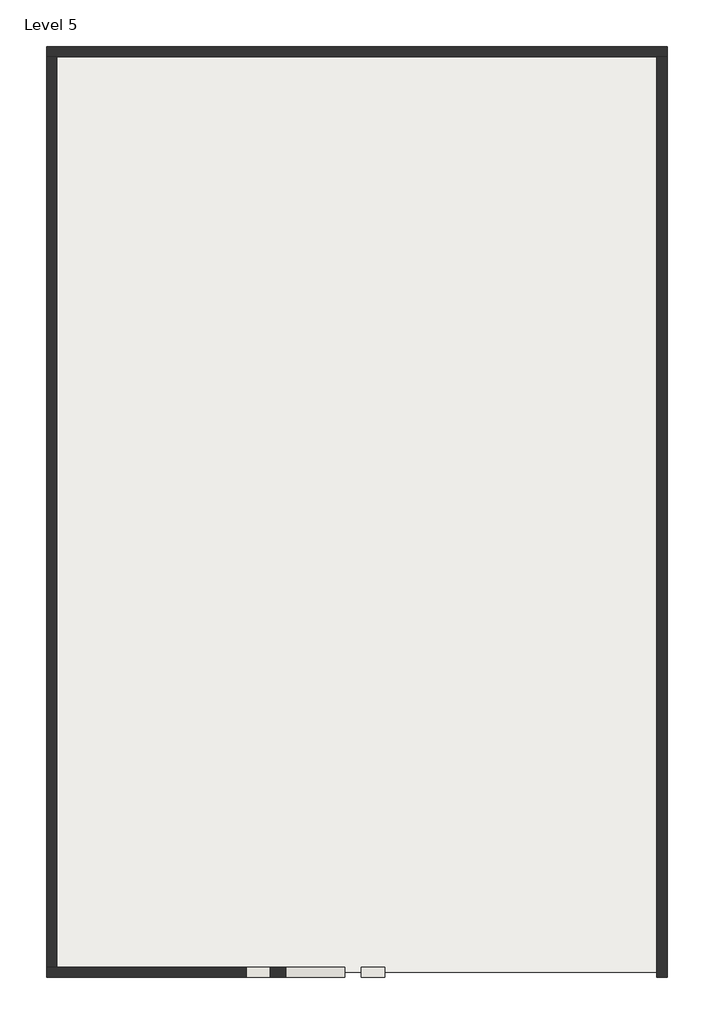
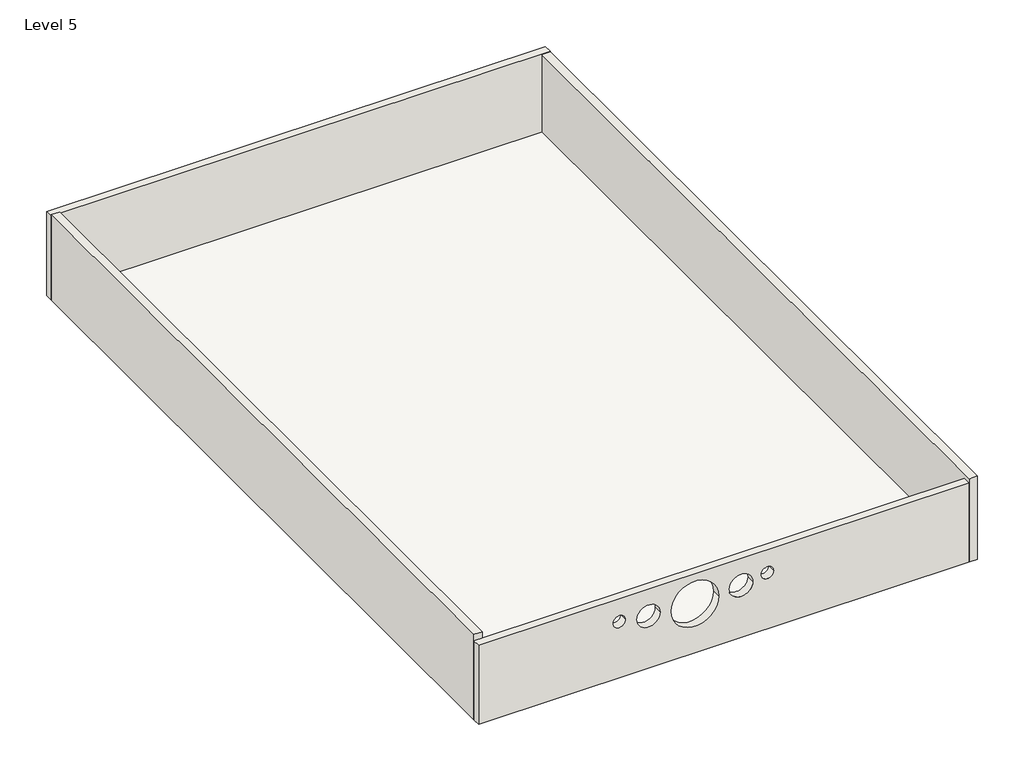
# One storey: 4 walls, 1 roof.
"""IFC4 building model written with IfcOpenShell, lengths in millimetres."""

from ifc_helpers import new_model, si_unit, frame, origin, place, context, project, spatial, polyline, circle_curve, outline, extrude, faceted_brep, element, save
from ifc_brep_helpers import plane_surface, revolved_surface, advanced_brep

model = new_model("IFC4")

# Units and contexts
model_context = context("Model", 3, world=origin())
ifc_project = project(units=[si_unit("LENGTHUNIT", "METRE", prefix="MILLI")], contexts=[model_context])

# Site, building, storey
site = spatial("IfcSite", under=ifc_project)
building = spatial("IfcBuilding", under=site)
storey = spatial("IfcBuildingStorey", under=building, Name="Level 5", Elevation=12192.0)

# Roof
placement = place(None, origin())
element("IfcRoof", 1, ObjectType="Generic - 12\"", at=placement, inside=storey, context=model_context, shape_type="SweptSolid", body=[
    extrude(outline(polyline([(-6134.0560205, 8955.7974079), (5981.7439795, 8955.7974079), (5981.7439795, -9323.5734342), (-6134.0560205, -9323.5734342), (-6134.0560205, 8955.7974079)])), frame((0.0, 0.0, 12192.0), z_axis=(0.0, 0.0, 1.0), x_axis=(1.0, 0.0, 0.0)), (0.0, 0.0, 1.0), 152.4),
])

# Walls
element("IfcWall", 2, ObjectType="Generic - 4.5\" p", at=placement, inside=storey, context=model_context, shape_type="Brep", body=[
    faceted_brep([(-6235.6560205, 8854.1974079, 12192.0), (-6032.4560205, 8854.1974079, 12192.0), (5880.1439795, 8854.1974079, 12192.0), (6083.3439795, 8854.1974079, 12192.0), (6083.3439795, 8854.1974079, 14367.9518297), (6083.3439795, 8854.1974079, 14383.5164153), (-6235.6560205, 8854.1974079, 14383.5164153), (-6235.6560205, 9057.3974079, 12192.0), (-6235.6560205, 9057.3974079, 14383.5164153), (6083.3439795, 9057.3974079, 14383.5164153), (6083.3439795, 9057.3974079, 12192.0)], [[[0, 1, 2, 3, 4, 5, 6]], [[7, 8, 9, 10]], [[3, 2, 1, 0, 7, 10]], [[6, 5, 9, 8]], [[5, 4, 3, 10, 9]], [[0, 6, 8, 7]]]),
])
element("IfcWall", 3, ObjectType="Generic - 4.5\" p", at=placement, inside=storey, context=model_context, shape_type="Brep", body=[
    faceted_brep([(5880.1439795, 8854.1974079, 12192.0), (5880.1439795, -9221.9734342, 12192.0), (5880.1439795, -9425.1734342, 12192.0), (5880.1439795, -9425.1734342, 14254.8371724), (5880.1439795, -9425.1734342, 14367.9518297), (5880.1439795, 8854.1974079, 14367.9518297), (6083.3439795, 8854.1974079, 12192.0), (6083.3439795, 8854.1974079, 14367.9518297), (6083.3439795, -9425.1734342, 14367.9518297), (6083.3439795, -9425.1734342, 12192.0)], [[[0, 1, 2, 3, 4, 5]], [[6, 7, 8, 9]], [[2, 1, 0, 6, 9]], [[5, 4, 8, 7]], [[0, 5, 7, 6]], [[4, 3, 2, 9, 8]]]),
])
element("IfcWall", 4, ObjectType="Generic - 4.5\" p", at=placement, inside=storey, context=model_context, shape_type="AdvancedBrep", body=[
    advanced_brep(
    [(5880.1439795, -9221.9734342, 12192.0), (-6032.4560205, -9221.9734342, 12192.0), (-6235.6560205, -9221.9734342, 12192.0), (-6235.6560205, -9221.9734342, 14254.8371724), (5880.1439795, -9221.9734342, 14254.8371724), (-1482.6330684, -9221.9734342, 13477.7338107), (-309.4573214, -9221.9734342, 13477.7338107), (-40.4133908, -9221.9734342, 13557.6568457), (534.323001, -9221.9734342, 13557.6568457), (743.9347645, -9221.9734342, 13663.3267882), (1048.7347645, -9221.9734342, 13663.3267882), (-2326.4133908, -9221.9734342, 13557.6568457), (-1751.676999, -9221.9734342, 13557.6568457), (-2913.6652355, -9221.9734342, 13663.3267882), (-2608.8652355, -9221.9734342, 13663.3267882), (5880.1439795, -9425.1734342, 12192.0), (5880.1439795, -9425.1734342, 14254.8371724), (-6235.6560205, -9425.1734342, 14254.8371724), (-6235.6560205, -9425.1734342, 12192.0), (-1482.6330684, -9425.1734342, 13477.7338107), (-309.4573214, -9425.1734342, 13477.7338107), (-40.4133908, -9425.1734342, 13557.6568457), (534.323001, -9425.1734342, 13557.6568457), (743.9347645, -9425.1734342, 13663.3267882), (1048.7347645, -9425.1734342, 13663.3267882), (-2326.4133908, -9425.1734342, 13557.6568457), (-1751.676999, -9425.1734342, 13557.6568457), (-2913.6652355, -9425.1734342, 13663.3267882), (-2608.8652355, -9425.1734342, 13663.3267882)],
    [
        (0, 1),
        (1, 2),
        (2, 3),
        (3, 4),
        (4, 0),
        (5, 6, circle_curve(frame((-896.0451949, -9221.9734342, 13477.7338107), z_axis=(0.0, -1.0, 0.0), x_axis=(1.0, 0.0, 0.0)), 586.5878735)),
        (6, 5, circle_curve(frame((-896.0451949, -9221.9734342, 13477.7338107), z_axis=(0.0, -1.0, 0.0), x_axis=(1.0, 0.0, 0.0)), 586.5878735)),
        (7, 8, circle_curve(frame((246.9548051, -9221.9734342, 13557.6568457), z_axis=(0.0, -1.0, 0.0), x_axis=(1.0, 0.0, 0.0)), 287.3681959)),
        (8, 7, circle_curve(frame((246.9548051, -9221.9734342, 13557.6568457), z_axis=(0.0, -1.0, 0.0), x_axis=(1.0, 0.0, 0.0)), 287.3681959)),
        (9, 10, circle_curve(frame((896.3347645, -9221.9734342, 13663.3267882), z_axis=(0.0, -1.0, 0.0), x_axis=(1.0, 0.0, 0.0)), 152.4)),
        (10, 9, circle_curve(frame((896.3347645, -9221.9734342, 13663.3267882), z_axis=(0.0, -1.0, 0.0), x_axis=(1.0, 0.0, 0.0)), 152.4)),
        (11, 12, circle_curve(frame((-2039.0451949, -9221.9734342, 13557.6568457), z_axis=(0.0, -1.0, 0.0), x_axis=(1.0, 0.0, 0.0)), 287.3681959)),
        (12, 11, circle_curve(frame((-2039.0451949, -9221.9734342, 13557.6568457), z_axis=(0.0, -1.0, 0.0), x_axis=(1.0, 0.0, 0.0)), 287.3681959)),
        (13, 14, circle_curve(frame((-2761.2652355, -9221.9734342, 13663.3267882), z_axis=(0.0, -1.0, 0.0), x_axis=(1.0, 0.0, 0.0)), 152.4)),
        (14, 13, circle_curve(frame((-2761.2652355, -9221.9734342, 13663.3267882), z_axis=(0.0, -1.0, 0.0), x_axis=(1.0, 0.0, 0.0)), 152.4)),
        (15, 16),
        (16, 17),
        (17, 18),
        (18, 15),
        (19, 20, circle_curve(frame((-896.0451949, -9425.1734342, 13477.7338107), z_axis=(0.0, 1.0, 0.0), x_axis=(1.0, 0.0, 0.0)), 586.5878735)),
        (20, 19, circle_curve(frame((-896.0451949, -9425.1734342, 13477.7338107), z_axis=(0.0, 1.0, 0.0), x_axis=(1.0, 0.0, 0.0)), 586.5878735)),
        (21, 22, circle_curve(frame((246.9548051, -9425.1734342, 13557.6568457), z_axis=(0.0, 1.0, 0.0), x_axis=(1.0, 0.0, 0.0)), 287.3681959)),
        (22, 21, circle_curve(frame((246.9548051, -9425.1734342, 13557.6568457), z_axis=(0.0, 1.0, 0.0), x_axis=(1.0, 0.0, 0.0)), 287.3681959)),
        (23, 24, circle_curve(frame((896.3347645, -9425.1734342, 13663.3267882), z_axis=(0.0, 1.0, 0.0), x_axis=(1.0, 0.0, 0.0)), 152.4)),
        (24, 23, circle_curve(frame((896.3347645, -9425.1734342, 13663.3267882), z_axis=(0.0, 1.0, 0.0), x_axis=(1.0, 0.0, 0.0)), 152.4)),
        (25, 26, circle_curve(frame((-2039.0451949, -9425.1734342, 13557.6568457), z_axis=(0.0, 1.0, 0.0), x_axis=(1.0, 0.0, 0.0)), 287.3681959)),
        (26, 25, circle_curve(frame((-2039.0451949, -9425.1734342, 13557.6568457), z_axis=(0.0, 1.0, 0.0), x_axis=(1.0, 0.0, 0.0)), 287.3681959)),
        (27, 28, circle_curve(frame((-2761.2652355, -9425.1734342, 13663.3267882), z_axis=(0.0, 1.0, 0.0), x_axis=(1.0, 0.0, 0.0)), 152.4)),
        (28, 27, circle_curve(frame((-2761.2652355, -9425.1734342, 13663.3267882), z_axis=(0.0, 1.0, 0.0), x_axis=(1.0, 0.0, 0.0)), 152.4)),
        (4, 16),
        (15, 0),
        (2, 18),
        (17, 3),
        (5, 19),
        (20, 6),
        (7, 21),
        (22, 8),
        (9, 23),
        (24, 10),
        (11, 25),
        (26, 12),
        (13, 27),
        (28, 14),
    ],
    [
        plane_surface(frame((5981.7439795, -9221.9734342, 12192.0), z_axis=(0.0, 1.0, 0.0), x_axis=(-1.0, 0.0, 0.0))),
        plane_surface(frame((5981.7439795, -9425.1734342, 12192.0), z_axis=(0.0, -1.0, 0.0), x_axis=(1.0, 0.0, 0.0))),
        plane_surface(frame((5880.1439795, 8955.7974079, 12192.0), z_axis=(1.0, 0.0, 0.0), x_axis=(0.0, -1.0, 0.0))),
        plane_surface(frame((-6235.6560205, -9323.5734342, 12192.0), z_axis=(-1.0, 0.0, 0.0), x_axis=(0.0, -1.0, 0.0))),
        plane_surface(frame((5981.7439795, -9221.9734342, 12192.0), z_axis=(0.0, 0.0, -1.0), x_axis=(0.0, -1.0, 0.0))),
        plane_surface(frame((-6134.0560205, -9221.9734342, 14254.8371724), z_axis=(0.0, 0.0, 1.0), x_axis=(0.0, -1.0, 0.0))),
        revolved_surface(polyline([(-309.45732139999996, -9425.1734342, 13477.7338107), (-309.45732139999996, -9221.9734342, 13477.7338107)]), (-896.0451949, -9323.5734342, 13477.7338107), (0.0, -1.0, 0.0)),
        revolved_surface(polyline([(534.323001, -9425.1734342, 13557.6568457), (534.323001, -9221.9734342, 13557.6568457)]), (246.9548051, -9323.5734342, 13557.6568457), (0.0, -1.0, 0.0)),
        revolved_surface(polyline([(1048.7347645, -9425.1734342, 13663.3267882), (1048.7347645, -9221.9734342, 13663.3267882)]), (896.3347645, -9323.5734342, 13663.3267882), (0.0, -1.0, 0.0)),
        revolved_surface(polyline([(-1751.676999, -9425.1734342, 13557.6568457), (-1751.676999, -9221.9734342, 13557.6568457)]), (-2039.0451949, -9323.5734342, 13557.6568457), (0.0, -1.0, 0.0)),
        revolved_surface(polyline([(-2608.8652355, -9425.1734342, 13663.3267882), (-2608.8652355, -9221.9734342, 13663.3267882)]), (-2761.2652355, -9323.5734342, 13663.3267882), (0.0, -1.0, 0.0)),
    ],
    [
        (0, [[1, 2, 3, 4, 5], [6, 7], [8, 9], [10, 11], [12, 13], [14, 15]]),
        (1, [[16, 17, 18, 19], [20, 21], [22, 23], [24, 25], [26, 27], [28, 29]]),
        (2, [[-5, 30, -16, 31]]),
        (3, [[-3, 32, -18, 33]]),
        (4, [[-2, -1, -31, -19, -32]]),
        (5, [[-4, -33, -17, -30]]),
        (6, [[-6, 34, -21, 35]]),
        (6, [[-7, -35, -20, -34]]),
        (7, [[-8, 36, -23, 37]]),
        (7, [[-9, -37, -22, -36]]),
        (8, [[-10, 38, -25, 39]]),
        (8, [[-11, -39, -24, -38]]),
        (9, [[-12, 40, -27, 41]]),
        (9, [[-13, -41, -26, -40]]),
        (10, [[-14, 42, -29, 43]]),
        (10, [[-15, -43, -28, -42]]),
    ],
),
])
element("IfcWall", 5, ObjectType="Generic - 4.5\" p", at=placement, inside=storey, context=model_context, shape_type="Brep", body=[
    faceted_brep([(-6032.4560205, -9221.9734342, 12192.0), (-6032.4560205, 8854.1974079, 12192.0), (-6032.4560205, 8854.1974079, 14423.3036487), (-6032.4560205, -9221.9734342, 14423.3036487), (-6235.6560205, -9221.9734342, 12192.0), (-6235.6560205, -9221.9734342, 14254.8371724), (-6235.6560205, -9221.9734342, 14423.3036487), (-6235.6560205, 8854.1974079, 14423.3036487), (-6235.6560205, 8854.1974079, 14383.5164153), (-6235.6560205, 8854.1974079, 12192.0)], [[[0, 1, 2, 3]], [[4, 5, 6, 7, 8, 9]], [[1, 0, 4, 9]], [[3, 2, 7, 6]], [[0, 3, 6, 5, 4]], [[2, 1, 9, 8, 7]]]),
])

save(model, "model.ifc")

# Revit data of these elements
# Type "Generic - 12\""
#   Assembly Code = "B1020"
#   Layers, outside or top first: 0' - 6" no material (function 1)
# Type "Generic - 4.5\" p"
#   Assembly Code = "B2010"
#   Layers, outside or top first: 0' - 8" no material (function 1)
# Element 1 (IfcRoof, "Generic - 12\"")
#   built-in parameter 1001705 = 40.5 (stored number, unit not read)
#   built-in parameter 1001710 = 33615
#   Phase Created = New Construction
#   Materials on its faces: "Default Roof", "Plywood, Sheathing"
# Element 2 (IfcWall, "Generic - 4.5\" p")
#   Top Offset = 0' - 0"
#   Base Offset = 0' - 0"
#   Unconnected Height = 7' - 2.28017"
#   wall height = 7' - 2.28017"
#   Phase Created = New Construction
#   Base Constraint = Level 5
#   Materials on its faces: "Plywood, Sheathing", "Default Wall", "Window Frame"
# Element 3 (IfcWall, "Generic - 4.5\" p")
#   Top Offset = 0' - 0"
#   Base Offset = 0' - 0"
#   Unconnected Height = 7' - 1.66739"
#   wall height = 7' - 1.66739"
#   Phase Created = New Construction
#   Base Constraint = Level 5
#   Materials on its faces: "Default Wall", "Plywood, Sheathing", "Parking Stripe"
# Element 4 (IfcWall, "Generic - 4.5\" p")
#   Top Offset = 0' - 0"
#   Base Offset = 0' - 0"
#   Unconnected Height = 6' - 9.21406"
#   wall height = 6' - 9.21406"
#   Phase Created = New Construction
#   Base Constraint = Level 5
#   Materials on its faces: "Default Wall", "Parking Stripe", "Plywood, Sheathing"
# Element 5 (IfcWall, "Generic - 4.5\" p")
#   Top Offset = 0' - 0"
#   Base Offset = 0' - 0"
#   Unconnected Height = 7' - 3.8466"
#   wall height = 7' - 3.8466"
#   Phase Created = New Construction
#   Base Constraint = Level 5
#   Materials on its faces: "Default Wall", "Plywood, Sheathing"
# Materials
#   "Default Roof": colour RGB 88 101 114, transparency 0, Cost = 0
#   "Plywood, Sheathing": class "Wood", colour RGB 212 179 113, transparency 0, Description = "Plywood, sheathing grade", Cost = 0
#   "Default Wall": colour RGB 128 128 128, transparency 0, Cost = 0
#   "Window Frame": colour RGB 249 249 249, transparency 0
#   "Parking Stripe": class "Paint", colour RGB 250 250 91, transparency 0, Cost = 0
